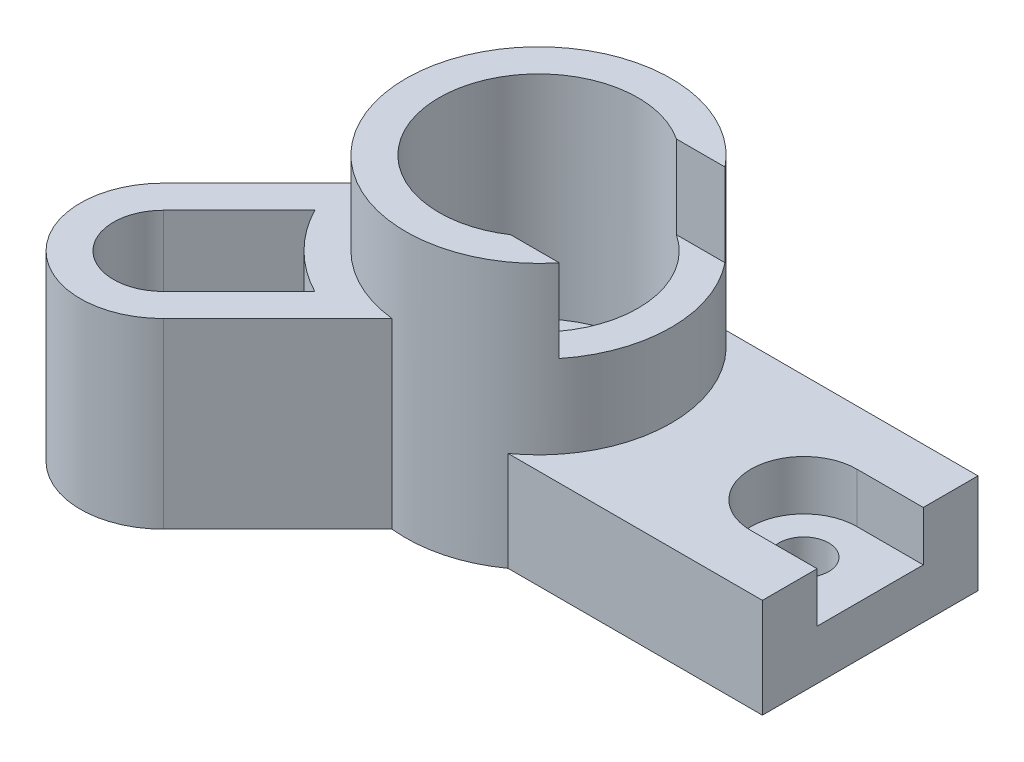
ISO-10303-21;
HEADER;
FILE_DESCRIPTION(('STEP AP214'),'2;1');
FILE_NAME('part.step','',(''),(''),'','','');
FILE_SCHEMA(('AUTOMOTIVE_DESIGN { 1 0 10303 214 1 1 1 1 }'));
ENDSEC;
DATA;
#1=APPLICATION_CONTEXT('core data for automotive mechanical design processes');
#2=APPLICATION_PROTOCOL_DEFINITION('international standard','automotive_design',2000,#1);
#3=PRODUCT_CONTEXT('',#1,'mechanical');
#4=PRODUCT('Part','Part','',(#3));
#5=PRODUCT_RELATED_PRODUCT_CATEGORY('part','',(#4));
#6=PRODUCT_DEFINITION_FORMATION('','',#4);
#7=PRODUCT_DEFINITION_CONTEXT('part definition',#1,'design');
#8=PRODUCT_DEFINITION('design','',#6,#7);
#9=PRODUCT_DEFINITION_SHAPE('','',#8);
#10=(LENGTH_UNIT() NAMED_UNIT(*) SI_UNIT(.MILLI.,.METRE.));
#11=(NAMED_UNIT(*) PLANE_ANGLE_UNIT() SI_UNIT($,.RADIAN.));
#12=(NAMED_UNIT(*) SI_UNIT($,.STERADIAN.) SOLID_ANGLE_UNIT());
#13=UNCERTAINTY_MEASURE_WITH_UNIT(LENGTH_MEASURE(1.E-05),#10,'distance_accuracy_value','');
#14=(GEOMETRIC_REPRESENTATION_CONTEXT(3) GLOBAL_UNCERTAINTY_ASSIGNED_CONTEXT((#13)) GLOBAL_UNIT_ASSIGNED_CONTEXT((#10,
#11,#12)) REPRESENTATION_CONTEXT('',''));
#15=CARTESIAN_POINT('',(0.,0.,0.));
#16=DIRECTION('',(0.,0.,1.));
#17=DIRECTION('',(1.,0.,0.));
#18=AXIS2_PLACEMENT_3D('',#15,#16,#17);
#19=CARTESIAN_POINT('',(0.,80.,0.));
#20=DIRECTION('',(0.,-1.,0.));
#21=DIRECTION('',(0.,0.,-1.));
#22=AXIS2_PLACEMENT_3D('',#19,#20,#21);
#23=CYLINDRICAL_SURFACE('',#22,40.);
#24=DIRECTION('',(0.,-1.,0.));
#25=VECTOR('',#24,1.);
#26=CARTESIAN_POINT('',(23.318447632722,30.,32.5));
#27=LINE('',#26,#25);
#28=CARTESIAN_POINT('',(23.318447632722,30.,32.5));
#29=VERTEX_POINT('',#28);
#30=CARTESIAN_POINT('',(23.318447632722,0.,32.5));
#31=VERTEX_POINT('',#30);
#32=EDGE_CURVE('E302',#29,#31,#27,.T.);
#33=ORIENTED_EDGE('',*,*,#32,.F.);
#34=CARTESIAN_POINT('',(0.,30.,0.));
#35=DIRECTION('',(0.,1.,0.));
#36=DIRECTION('',(0.,0.,1.));
#37=AXIS2_PLACEMENT_3D('',#34,#35,#36);
#38=CIRCLE('',#37,40.);
#39=CARTESIAN_POINT('',(23.318447632722,30.,-32.5));
#40=VERTEX_POINT('',#39);
#41=EDGE_CURVE('E279',#29,#40,#38,.T.);
#42=ORIENTED_EDGE('',*,*,#41,.T.);
#43=DIRECTION('',(0.,-1.,0.));
#44=VECTOR('',#43,1.);
#45=CARTESIAN_POINT('',(23.318447632722,30.,-32.5));
#46=LINE('',#45,#44);
#47=CARTESIAN_POINT('',(23.318447632722,0.,-32.5));
#48=VERTEX_POINT('',#47);
#49=EDGE_CURVE('E289',#40,#48,#46,.T.);
#50=ORIENTED_EDGE('',*,*,#49,.T.);
#51=CARTESIAN_POINT('',(0.,0.,0.));
#52=DIRECTION('',(0.,1.,0.));
#53=DIRECTION('',(0.,0.,1.));
#54=AXIS2_PLACEMENT_3D('',#51,#52,#53);
#55=CIRCLE('',#54,40.);
#56=CARTESIAN_POINT('',(-39.7570716954833,0.,4.40173263615613));
#57=VERTEX_POINT('',#56);
#58=EDGE_CURVE('E332',#48,#57,#55,.T.);
#59=ORIENTED_EDGE('',*,*,#58,.T.);
#60=DIRECTION('',(0.,-1.,0.));
#61=VECTOR('',#60,1.);
#62=CARTESIAN_POINT('',(-39.7570716954833,55.,4.40173263615613));
#63=LINE('',#62,#61);
#64=CARTESIAN_POINT('',(-39.7570716954833,55.,4.40173263615613));
#65=VERTEX_POINT('',#64);
#66=EDGE_CURVE('E335',#65,#57,#63,.T.);
#67=ORIENTED_EDGE('',*,*,#66,.F.);
#68=CARTESIAN_POINT('',(0.,55.,0.));
#69=DIRECTION('',(0.,1.,0.));
#70=DIRECTION('',(0.,0.,1.));
#71=AXIS2_PLACEMENT_3D('',#68,#69,#70);
#72=CIRCLE('',#71,40.);
#73=CARTESIAN_POINT('',(-4.40173263615573,55.,39.7570716954833));
#74=VERTEX_POINT('',#73);
#75=EDGE_CURVE('E310',#65,#74,#72,.T.);
#76=ORIENTED_EDGE('',*,*,#75,.T.);
#77=DIRECTION('',(0.,-1.,0.));
#78=VECTOR('',#77,1.);
#79=CARTESIAN_POINT('',(-4.40173263615573,55.,39.7570716954833));
#80=LINE('',#79,#78);
#81=CARTESIAN_POINT('',(-4.40173263615573,0.,39.7570716954833));
#82=VERTEX_POINT('',#81);
#83=EDGE_CURVE('E316',#74,#82,#80,.T.);
#84=ORIENTED_EDGE('',*,*,#83,.T.);
#85=EDGE_CURVE('E42',#82,#31,#55,.T.);
#86=ORIENTED_EDGE('',*,*,#85,.T.);
#87=EDGE_LOOP('',(#33,#42,#50,#59,#67,#76,#84,#86));
#88=FACE_BOUND('',#87,.T.);
#89=DIRECTION('',(0.,-1.,0.));
#90=VECTOR('',#89,1.);
#91=CARTESIAN_POINT('',(31.224989991992,80.001,25.));
#92=LINE('',#91,#90);
#93=CARTESIAN_POINT('',(31.224989991992,80.,25.));
#94=VERTEX_POINT('',#93);
#95=CARTESIAN_POINT('',(31.224989991992,55.,25.));
#96=VERTEX_POINT('',#95);
#97=EDGE_CURVE('E220',#94,#96,#92,.T.);
#98=ORIENTED_EDGE('',*,*,#97,.F.);
#99=CARTESIAN_POINT('',(0.,80.,0.));
#100=DIRECTION('',(0.,1.,0.));
#101=DIRECTION('',(0.,0.,1.));
#102=AXIS2_PLACEMENT_3D('',#99,#100,#101);
#103=CIRCLE('',#102,40.);
#104=CARTESIAN_POINT('',(31.224989991992,80.,-25.));
#105=VERTEX_POINT('',#104);
#106=EDGE_CURVE('E11',#105,#94,#103,.T.);
#107=ORIENTED_EDGE('',*,*,#106,.F.);
#108=DIRECTION('',(0.,-1.,0.));
#109=VECTOR('',#108,1.);
#110=CARTESIAN_POINT('',(31.224989991992,80.001,-25.));
#111=LINE('',#110,#109);
#112=CARTESIAN_POINT('',(31.224989991992,55.,-25.));
#113=VERTEX_POINT('',#112);
#114=EDGE_CURVE('E213',#105,#113,#111,.T.);
#115=ORIENTED_EDGE('',*,*,#114,.T.);
#116=CARTESIAN_POINT('',(0.,55.,0.));
#117=DIRECTION('',(0.,1.,0.));
#118=DIRECTION('',(0.,0.,1.));
#119=AXIS2_PLACEMENT_3D('',#116,#117,#118);
#120=CIRCLE('',#119,40.);
#121=EDGE_CURVE('E202',#96,#113,#120,.T.);
#122=ORIENTED_EDGE('',*,*,#121,.F.);
#123=EDGE_LOOP('',(#98,#107,#115,#122));
#124=FACE_BOUND('',#123,.T.);
#125=ADVANCED_FACE('F41',(#88,#124),#23,.T.);
#126=CARTESIAN_POINT('',(0.,80.,0.));
#127=DIRECTION('',(0.,1.,0.));
#128=DIRECTION('',(0.,0.,1.));
#129=AXIS2_PLACEMENT_3D('',#126,#127,#128);
#130=PLANE('',#129);
#131=CARTESIAN_POINT('',(0.,80.,0.));
#132=DIRECTION('',(0.,1.,0.));
#133=DIRECTION('',(0.,0.,1.));
#134=AXIS2_PLACEMENT_3D('',#131,#132,#133);
#135=CIRCLE('',#134,30.);
#136=CARTESIAN_POINT('',(16.583123951777,80.,-25.));
#137=VERTEX_POINT('',#136);
#138=CARTESIAN_POINT('',(16.583123951777,80.,25.));
#139=VERTEX_POINT('',#138);
#140=EDGE_CURVE('E176',#137,#139,#135,.T.);
#141=ORIENTED_EDGE('',*,*,#140,.F.);
#142=DIRECTION('',(1.,0.,0.));
#143=VECTOR('',#142,1.);
#144=CARTESIAN_POINT('',(16.583123951777,80.,-25.));
#145=LINE('',#144,#143);
#146=EDGE_CURVE('E205',#137,#105,#145,.T.);
#147=ORIENTED_EDGE('',*,*,#146,.T.);
#148=ORIENTED_EDGE('',*,*,#106,.T.);
#149=DIRECTION('',(1.,0.,0.));
#150=VECTOR('',#149,1.);
#151=CARTESIAN_POINT('',(16.583123951777,80.,25.));
#152=LINE('',#151,#150);
#153=EDGE_CURVE('E195',#139,#94,#152,.T.);
#154=ORIENTED_EDGE('',*,*,#153,.F.);
#155=EDGE_LOOP('',(#141,#147,#148,#154));
#156=FACE_BOUND('',#155,.T.);
#157=ADVANCED_FACE('F199',(#156),#130,.T.);
#158=CARTESIAN_POINT('',(100.,30.,0.));
#159=DIRECTION('',(1.,0.,0.));
#160=DIRECTION('',(0.,0.,-1.));
#161=AXIS2_PLACEMENT_3D('',#158,#159,#160);
#162=PLANE('',#161);
#163=DIRECTION('',(0.,0.,1.));
#164=VECTOR('',#163,1.);
#165=CARTESIAN_POINT('',(100.,15.,0.));
#166=LINE('',#165,#164);
#167=CARTESIAN_POINT('',(100.,15.,-16.));
#168=VERTEX_POINT('',#167);
#169=CARTESIAN_POINT('',(100.,15.,16.));
#170=VERTEX_POINT('',#169);
#171=EDGE_CURVE('E225',#168,#170,#166,.T.);
#172=ORIENTED_EDGE('',*,*,#171,.T.);
#173=DIRECTION('',(0.,1.,0.));
#174=VECTOR('',#173,1.);
#175=CARTESIAN_POINT('',(100.,15.,16.));
#176=LINE('',#175,#174);
#177=CARTESIAN_POINT('',(100.,30.,16.));
#178=VERTEX_POINT('',#177);
#179=EDGE_CURVE('E241',#170,#178,#176,.T.);
#180=ORIENTED_EDGE('',*,*,#179,.T.);
#181=DIRECTION('',(0.,0.,1.));
#182=VECTOR('',#181,1.);
#183=CARTESIAN_POINT('',(100.,30.,0.));
#184=LINE('',#183,#182);
#185=CARTESIAN_POINT('',(100.,30.,32.5));
#186=VERTEX_POINT('',#185);
#187=EDGE_CURVE('E283',#178,#186,#184,.T.);
#188=ORIENTED_EDGE('',*,*,#187,.T.);
#189=DIRECTION('',(0.,-1.,0.));
#190=VECTOR('',#189,1.);
#191=CARTESIAN_POINT('',(100.,30.,32.5));
#192=LINE('',#191,#190);
#193=CARTESIAN_POINT('',(100.,0.,32.5));
#194=VERTEX_POINT('',#193);
#195=EDGE_CURVE('E305',#186,#194,#192,.T.);
#196=ORIENTED_EDGE('',*,*,#195,.T.);
#197=DIRECTION('',(0.,0.,1.));
#198=VECTOR('',#197,1.);
#199=CARTESIAN_POINT('',(100.,0.,0.));
#200=LINE('',#199,#198);
#201=CARTESIAN_POINT('',(100.,0.,-32.5));
#202=VERTEX_POINT('',#201);
#203=EDGE_CURVE('E291',#202,#194,#200,.T.);
#204=ORIENTED_EDGE('',*,*,#203,.F.);
#205=DIRECTION('',(0.,-1.,0.));
#206=VECTOR('',#205,1.);
#207=CARTESIAN_POINT('',(100.,30.,-32.5));
#208=LINE('',#207,#206);
#209=CARTESIAN_POINT('',(100.,30.,-32.5));
#210=VERTEX_POINT('',#209);
#211=EDGE_CURVE('E297',#210,#202,#208,.T.);
#212=ORIENTED_EDGE('',*,*,#211,.F.);
#213=CARTESIAN_POINT('',(100.,30.,-16.));
#214=VERTEX_POINT('',#213);
#215=EDGE_CURVE('E282',#210,#214,#184,.T.);
#216=ORIENTED_EDGE('',*,*,#215,.T.);
#217=DIRECTION('',(0.,1.,0.));
#218=VECTOR('',#217,1.);
#219=CARTESIAN_POINT('',(100.,15.,-16.));
#220=LINE('',#219,#218);
#221=EDGE_CURVE('E242',#168,#214,#220,.T.);
#222=ORIENTED_EDGE('',*,*,#221,.F.);
#223=EDGE_LOOP('',(#172,#180,#188,#196,#204,#212,#216,#222));
#224=FACE_BOUND('',#223,.T.);
#225=ADVANCED_FACE('F386',(#224),#162,.T.);
#226=CARTESIAN_POINT('',(0.,30.,0.));
#227=DIRECTION('',(0.,1.,0.));
#228=DIRECTION('',(0.,0.,1.));
#229=AXIS2_PLACEMENT_3D('',#226,#227,#228);
#230=PLANE('',#229);
#231=CARTESIAN_POINT('',(80.,30.,0.));
#232=DIRECTION('',(0.,1.,0.));
#233=DIRECTION('',(0.,0.,1.));
#234=AXIS2_PLACEMENT_3D('',#231,#232,#233);
#235=CIRCLE('',#234,16.);
#236=CARTESIAN_POINT('',(80.,30.,-16.));
#237=VERTEX_POINT('',#236);
#238=CARTESIAN_POINT('',(80.,30.,16.));
#239=VERTEX_POINT('',#238);
#240=EDGE_CURVE('E223',#237,#239,#235,.T.);
#241=ORIENTED_EDGE('',*,*,#240,.F.);
#242=DIRECTION('',(1.,0.,0.));
#243=VECTOR('',#242,1.);
#244=CARTESIAN_POINT('',(0.,30.,-16.));
#245=LINE('',#244,#243);
#246=EDGE_CURVE('E54',#237,#214,#245,.T.);
#247=ORIENTED_EDGE('',*,*,#246,.T.);
#248=ORIENTED_EDGE('',*,*,#215,.F.);
#249=DIRECTION('',(1.,0.,0.));
#250=VECTOR('',#249,1.);
#251=CARTESIAN_POINT('',(0.,30.,-32.4999999999999));
#252=LINE('',#251,#250);
#253=EDGE_CURVE('E290',#40,#210,#252,.T.);
#254=ORIENTED_EDGE('',*,*,#253,.F.);
#255=ORIENTED_EDGE('',*,*,#41,.F.);
#256=DIRECTION('',(1.,0.,0.));
#257=VECTOR('',#256,1.);
#258=CARTESIAN_POINT('',(0.,30.,32.5));
#259=LINE('',#258,#257);
#260=EDGE_CURVE('E278',#29,#186,#259,.T.);
#261=ORIENTED_EDGE('',*,*,#260,.T.);
#262=ORIENTED_EDGE('',*,*,#187,.F.);
#263=DIRECTION('',(1.,0.,0.));
#264=VECTOR('',#263,1.);
#265=CARTESIAN_POINT('',(0.,30.,16.));
#266=LINE('',#265,#264);
#267=EDGE_CURVE('E234',#239,#178,#266,.T.);
#268=ORIENTED_EDGE('',*,*,#267,.F.);
#269=EDGE_LOOP('',(#241,#247,#248,#254,#255,#261,#262,#268));
#270=FACE_BOUND('',#269,.T.);
#271=ADVANCED_FACE('F357',(#270),#230,.T.);
#272=CARTESIAN_POINT('',(0.,0.,0.));
#273=DIRECTION('',(0.,1.,0.));
#274=DIRECTION('',(0.,0.,1.));
#275=AXIS2_PLACEMENT_3D('',#272,#273,#274);
#276=PLANE('',#275);
#277=CARTESIAN_POINT('',(-56.5685424949235,0.,56.5685424949241));
#278=DIRECTION('',(0.,-1.,0.));
#279=DIRECTION('',(0.,0.,-1.));
#280=AXIS2_PLACEMENT_3D('',#277,#278,#279);
#281=CIRCLE('',#280,10.);
#282=CARTESIAN_POINT('',(-56.5685424949235,0.,46.5685424949241));
#283=VERTEX_POINT('',#282);
#284=EDGE_CURVE('E186',#283,#283,#281,.T.);
#285=ORIENTED_EDGE('',*,*,#284,.F.);
#286=EDGE_LOOP('',(#285));
#287=FACE_BOUND('',#286,.T.);
#288=CARTESIAN_POINT('',(80.,0.,0.));
#289=DIRECTION('',(0.,-1.,0.));
#290=DIRECTION('',(0.,0.,-1.));
#291=AXIS2_PLACEMENT_3D('',#288,#289,#290);
#292=CIRCLE('',#291,7.5);
#293=CARTESIAN_POINT('',(80.,0.,-7.5));
#294=VERTEX_POINT('',#293);
#295=EDGE_CURVE('E411',#294,#294,#292,.T.);
#296=ORIENTED_EDGE('',*,*,#295,.F.);
#297=EDGE_LOOP('',(#296));
#298=FACE_BOUND('',#297,.T.);
#299=CARTESIAN_POINT('',(0.,0.,0.));
#300=DIRECTION('',(0.,-1.,0.));
#301=DIRECTION('',(0.,0.,-1.));
#302=AXIS2_PLACEMENT_3D('',#299,#300,#301);
#303=CIRCLE('',#302,20.);
#304=CARTESIAN_POINT('',(0.,0.,-20.));
#305=VERTEX_POINT('',#304);
#306=EDGE_CURVE('E412',#305,#305,#303,.T.);
#307=ORIENTED_EDGE('',*,*,#306,.F.);
#308=EDGE_LOOP('',(#307));
#309=FACE_BOUND('',#308,.T.);
#310=ORIENTED_EDGE('',*,*,#85,.F.);
#311=DIRECTION('',(0.707106781186544,0.,-0.707106781186551));
#312=VECTOR('',#311,1.);
#313=CARTESIAN_POINT('',(17.6776695296638,0.,17.6776695296636));
#314=LINE('',#313,#312);
#315=CARTESIAN_POINT('',(-38.8908729652597,0.,74.2462120245877));
#316=VERTEX_POINT('',#315);
#317=EDGE_CURVE('E311',#316,#82,#314,.T.);
#318=ORIENTED_EDGE('',*,*,#317,.F.);
#319=CARTESIAN_POINT('',(-56.5685424949235,0.,56.5685424949241));
#320=DIRECTION('',(0.,1.,0.));
#321=DIRECTION('',(0.,0.,1.));
#322=AXIS2_PLACEMENT_3D('',#319,#320,#321);
#323=CIRCLE('',#322,25.);
#324=CARTESIAN_POINT('',(-74.2462120245873,0.,38.8908729652605));
#325=VERTEX_POINT('',#324);
#326=EDGE_CURVE('E321',#325,#316,#323,.T.);
#327=ORIENTED_EDGE('',*,*,#326,.F.);
#328=DIRECTION('',(0.707106781186544,0.,-0.707106781186551));
#329=VECTOR('',#328,1.);
#330=CARTESIAN_POINT('',(-17.6776695296638,0.,-17.6776695296636));
#331=LINE('',#330,#329);
#332=EDGE_CURVE('E306',#325,#57,#331,.T.);
#333=ORIENTED_EDGE('',*,*,#332,.T.);
#334=ORIENTED_EDGE('',*,*,#58,.F.);
#335=DIRECTION('',(1.,0.,0.));
#336=VECTOR('',#335,1.);
#337=CARTESIAN_POINT('',(0.,0.,-32.4999999999999));
#338=LINE('',#337,#336);
#339=EDGE_CURVE('E277',#48,#202,#338,.T.);
#340=ORIENTED_EDGE('',*,*,#339,.T.);
#341=ORIENTED_EDGE('',*,*,#203,.T.);
#342=DIRECTION('',(1.,0.,0.));
#343=VECTOR('',#342,1.);
#344=CARTESIAN_POINT('',(0.,0.,32.5));
#345=LINE('',#344,#343);
#346=EDGE_CURVE('E269',#31,#194,#345,.T.);
#347=ORIENTED_EDGE('',*,*,#346,.F.);
#348=EDGE_LOOP('',(#310,#318,#327,#333,#334,#340,#341,#347));
#349=FACE_BOUND('',#348,.T.);
#350=ADVANCED_FACE('F350',(#287,#298,#309,#349),#276,.F.);
#351=CARTESIAN_POINT('',(-17.6776695296638,55.,-17.6776695296636));
#352=DIRECTION('',(-0.707106781186551,0.,-0.707106781186544));
#353=DIRECTION('',(-0.707106781186544,0.,0.707106781186551));
#354=AXIS2_PLACEMENT_3D('',#351,#352,#353);
#355=PLANE('',#354);
#356=ORIENTED_EDGE('',*,*,#332,.F.);
#357=DIRECTION('',(0.,-1.,0.));
#358=VECTOR('',#357,1.);
#359=CARTESIAN_POINT('',(-74.2462120245873,55.,38.8908729652605));
#360=LINE('',#359,#358);
#361=CARTESIAN_POINT('',(-74.2462120245873,55.,38.8908729652605));
#362=VERTEX_POINT('',#361);
#363=EDGE_CURVE('E329',#362,#325,#360,.T.);
#364=ORIENTED_EDGE('',*,*,#363,.F.);
#365=DIRECTION('',(0.707106781186544,0.,-0.707106781186551));
#366=VECTOR('',#365,1.);
#367=CARTESIAN_POINT('',(-17.6776695296638,55.,-17.6776695296636));
#368=LINE('',#367,#366);
#369=EDGE_CURVE('E309',#362,#65,#368,.T.);
#370=ORIENTED_EDGE('',*,*,#369,.T.);
#371=ORIENTED_EDGE('',*,*,#66,.T.);
#372=EDGE_LOOP('',(#356,#364,#370,#371));
#373=FACE_BOUND('',#372,.T.);
#374=ADVANCED_FACE('F363',(#373),#355,.T.);
#375=CARTESIAN_POINT('',(-56.5685424949235,55.,56.5685424949241));
#376=DIRECTION('',(0.,-1.,0.));
#377=DIRECTION('',(0.,0.,-1.));
#378=AXIS2_PLACEMENT_3D('',#375,#376,#377);
#379=CYLINDRICAL_SURFACE('',#378,25.);
#380=ORIENTED_EDGE('',*,*,#326,.T.);
#381=DIRECTION('',(0.,-1.,0.));
#382=VECTOR('',#381,1.);
#383=CARTESIAN_POINT('',(-38.8908729652597,55.,74.2462120245877));
#384=LINE('',#383,#382);
#385=CARTESIAN_POINT('',(-38.8908729652597,55.,74.2462120245877));
#386=VERTEX_POINT('',#385);
#387=EDGE_CURVE('E330',#386,#316,#384,.T.);
#388=ORIENTED_EDGE('',*,*,#387,.F.);
#389=CARTESIAN_POINT('',(-56.5685424949235,55.,56.5685424949241));
#390=DIRECTION('',(0.,1.,0.));
#391=DIRECTION('',(0.,0.,1.));
#392=AXIS2_PLACEMENT_3D('',#389,#390,#391);
#393=CIRCLE('',#392,25.);
#394=EDGE_CURVE('E313',#362,#386,#393,.T.);
#395=ORIENTED_EDGE('',*,*,#394,.F.);
#396=ORIENTED_EDGE('',*,*,#363,.T.);
#397=EDGE_LOOP('',(#380,#388,#395,#396));
#398=FACE_BOUND('',#397,.T.);
#399=ADVANCED_FACE('F366',(#398),#379,.T.);
#400=CARTESIAN_POINT('',(17.6776695296638,55.,17.6776695296636));
#401=DIRECTION('',(-0.707106781186552,0.,-0.707106781186544));
#402=DIRECTION('',(-0.707106781186544,0.,0.707106781186551));
#403=AXIS2_PLACEMENT_3D('',#400,#401,#402);
#404=PLANE('',#403);
#405=ORIENTED_EDGE('',*,*,#317,.T.);
#406=ORIENTED_EDGE('',*,*,#83,.F.);
#407=DIRECTION('',(0.707106781186544,0.,-0.707106781186551));
#408=VECTOR('',#407,1.);
#409=CARTESIAN_POINT('',(17.6776695296638,55.,17.6776695296636));
#410=LINE('',#409,#408);
#411=EDGE_CURVE('E317',#386,#74,#410,.T.);
#412=ORIENTED_EDGE('',*,*,#411,.F.);
#413=ORIENTED_EDGE('',*,*,#387,.T.);
#414=EDGE_LOOP('',(#405,#406,#412,#413));
#415=FACE_BOUND('',#414,.T.);
#416=ADVANCED_FACE('F371',(#415),#404,.F.);
#417=CARTESIAN_POINT('',(0.,55.,0.));
#418=DIRECTION('',(0.,1.,0.));
#419=DIRECTION('',(0.,0.,1.));
#420=AXIS2_PLACEMENT_3D('',#417,#418,#419);
#421=PLANE('',#420);
#422=DIRECTION('',(-0.707106781186544,0.,0.707106781186551));
#423=VECTOR('',#422,1.);
#424=CARTESIAN_POINT('',(-10.6066017177983,55.,-10.6066017177982));
#425=LINE('',#424,#423);
#426=CARTESIAN_POINT('',(-44.3334456258782,55.,23.1202421902821));
#427=VERTEX_POINT('',#426);
#428=CARTESIAN_POINT('',(-67.1751442127218,55.,45.9619407771259));
#429=VERTEX_POINT('',#428);
#430=EDGE_CURVE('E65',#427,#429,#425,.T.);
#431=ORIENTED_EDGE('',*,*,#430,.F.);
#432=CARTESIAN_POINT('',(0.,55.,0.));
#433=DIRECTION('',(0.,1.,0.));
#434=DIRECTION('',(0.,0.,1.));
#435=AXIS2_PLACEMENT_3D('',#432,#433,#434);
#436=CIRCLE('',#435,50.);
#437=CARTESIAN_POINT('',(-23.1202421902817,55.,44.3334456258784));
#438=VERTEX_POINT('',#437);
#439=EDGE_CURVE('E249',#427,#438,#436,.T.);
#440=ORIENTED_EDGE('',*,*,#439,.T.);
#441=DIRECTION('',(0.707106781186544,0.,-0.707106781186551));
#442=VECTOR('',#441,1.);
#443=CARTESIAN_POINT('',(10.6066017177983,55.,10.6066017177981));
#444=LINE('',#443,#442);
#445=CARTESIAN_POINT('',(-45.9619407771252,55.,67.1751442127222));
#446=VERTEX_POINT('',#445);
#447=EDGE_CURVE('E263',#446,#438,#444,.T.);
#448=ORIENTED_EDGE('',*,*,#447,.F.);
#449=CARTESIAN_POINT('',(-56.5685424949235,55.,56.5685424949241));
#450=DIRECTION('',(0.,1.,0.));
#451=DIRECTION('',(0.,0.,1.));
#452=AXIS2_PLACEMENT_3D('',#449,#450,#451);
#453=CIRCLE('',#452,15.);
#454=EDGE_CURVE('E257',#429,#446,#453,.T.);
#455=ORIENTED_EDGE('',*,*,#454,.F.);
#456=EDGE_LOOP('',(#431,#440,#448,#455));
#457=FACE_BOUND('',#456,.T.);
#458=ORIENTED_EDGE('',*,*,#75,.F.);
#459=ORIENTED_EDGE('',*,*,#369,.F.);
#460=ORIENTED_EDGE('',*,*,#394,.T.);
#461=ORIENTED_EDGE('',*,*,#411,.T.);
#462=EDGE_LOOP('',(#458,#459,#460,#461));
#463=FACE_BOUND('',#462,.T.);
#464=ADVANCED_FACE('F367',(#457,#463),#421,.T.);
#465=CARTESIAN_POINT('',(0.,30.,32.5));
#466=DIRECTION('',(0.,0.,-1.));
#467=DIRECTION('',(-1.,0.,0.));
#468=AXIS2_PLACEMENT_3D('',#465,#466,#467);
#469=PLANE('',#468);
#470=ORIENTED_EDGE('',*,*,#346,.T.);
#471=ORIENTED_EDGE('',*,*,#195,.F.);
#472=ORIENTED_EDGE('',*,*,#260,.F.);
#473=ORIENTED_EDGE('',*,*,#32,.T.);
#474=EDGE_LOOP('',(#470,#471,#472,#473));
#475=FACE_BOUND('',#474,.T.);
#476=ADVANCED_FACE('F355',(#475),#469,.F.);
#477=CARTESIAN_POINT('',(0.,30.,-32.4999999999999));
#478=DIRECTION('',(0.,0.,-1.));
#479=DIRECTION('',(-1.,0.,0.));
#480=AXIS2_PLACEMENT_3D('',#477,#478,#479);
#481=PLANE('',#480);
#482=ORIENTED_EDGE('',*,*,#339,.F.);
#483=ORIENTED_EDGE('',*,*,#49,.F.);
#484=ORIENTED_EDGE('',*,*,#253,.T.);
#485=ORIENTED_EDGE('',*,*,#211,.T.);
#486=EDGE_LOOP('',(#482,#483,#484,#485));
#487=FACE_BOUND('',#486,.T.);
#488=ADVANCED_FACE('F472',(#487),#481,.T.);
#489=CARTESIAN_POINT('',(-10.6066017177983,30.,-10.6066017177982));
#490=DIRECTION('',(-0.707106781186551,0.,-0.707106781186544));
#491=DIRECTION('',(-0.707106781186544,0.,0.707106781186551));
#492=AXIS2_PLACEMENT_3D('',#489,#490,#491);
#493=PLANE('',#492);
#494=ORIENTED_EDGE('',*,*,#430,.T.);
#495=DIRECTION('',(0.,1.,0.));
#496=VECTOR('',#495,1.);
#497=CARTESIAN_POINT('',(-67.1751442127218,30.,45.9619407771259));
#498=LINE('',#497,#496);
#499=CARTESIAN_POINT('',(-67.1751442127218,30.,45.9619407771259));
#500=VERTEX_POINT('',#499);
#501=EDGE_CURVE('E260',#500,#429,#498,.T.);
#502=ORIENTED_EDGE('',*,*,#501,.F.);
#503=DIRECTION('',(-0.707106781186544,0.,0.707106781186551));
#504=VECTOR('',#503,1.);
#505=CARTESIAN_POINT('',(-10.6066017177983,30.,-10.6066017177982));
#506=LINE('',#505,#504);
#507=CARTESIAN_POINT('',(-44.3334456258782,30.,23.1202421902821));
#508=VERTEX_POINT('',#507);
#509=EDGE_CURVE('E246',#508,#500,#506,.T.);
#510=ORIENTED_EDGE('',*,*,#509,.F.);
#511=DIRECTION('',(0.,1.,0.));
#512=VECTOR('',#511,1.);
#513=CARTESIAN_POINT('',(-44.3334456258782,30.,23.1202421902821));
#514=LINE('',#513,#512);
#515=EDGE_CURVE('E268',#508,#427,#514,.T.);
#516=ORIENTED_EDGE('',*,*,#515,.T.);
#517=EDGE_LOOP('',(#494,#502,#510,#516));
#518=FACE_BOUND('',#517,.T.);
#519=ADVANCED_FACE('F467',(#518),#493,.F.);
#520=CARTESIAN_POINT('',(0.,30.,0.));
#521=DIRECTION('',(0.,1.,0.));
#522=DIRECTION('',(0.,0.,1.));
#523=AXIS2_PLACEMENT_3D('',#520,#521,#522);
#524=CYLINDRICAL_SURFACE('',#523,50.);
#525=ORIENTED_EDGE('',*,*,#439,.F.);
#526=ORIENTED_EDGE('',*,*,#515,.F.);
#527=CARTESIAN_POINT('',(0.,30.,0.));
#528=DIRECTION('',(0.,1.,0.));
#529=DIRECTION('',(0.,0.,1.));
#530=AXIS2_PLACEMENT_3D('',#527,#528,#529);
#531=CIRCLE('',#530,50.);
#532=CARTESIAN_POINT('',(-23.1202421902817,30.,44.3334456258784));
#533=VERTEX_POINT('',#532);
#534=EDGE_CURVE('E259',#508,#533,#531,.T.);
#535=ORIENTED_EDGE('',*,*,#534,.T.);
#536=DIRECTION('',(0.,1.,0.));
#537=VECTOR('',#536,1.);
#538=CARTESIAN_POINT('',(-23.1202421902817,30.,44.3334456258784));
#539=LINE('',#538,#537);
#540=EDGE_CURVE('E272',#533,#438,#539,.T.);
#541=ORIENTED_EDGE('',*,*,#540,.T.);
#542=EDGE_LOOP('',(#525,#526,#535,#541));
#543=FACE_BOUND('',#542,.T.);
#544=ADVANCED_FACE('F465',(#543),#524,.T.);
#545=CARTESIAN_POINT('',(10.6066017177983,30.,10.6066017177981));
#546=DIRECTION('',(0.707106781186551,0.,0.707106781186544));
#547=DIRECTION('',(0.707106781186544,0.,-0.707106781186551));
#548=AXIS2_PLACEMENT_3D('',#545,#546,#547);
#549=PLANE('',#548);
#550=ORIENTED_EDGE('',*,*,#447,.T.);
#551=ORIENTED_EDGE('',*,*,#540,.F.);
#552=DIRECTION('',(0.707106781186544,0.,-0.707106781186551));
#553=VECTOR('',#552,1.);
#554=CARTESIAN_POINT('',(10.6066017177983,30.,10.6066017177981));
#555=LINE('',#554,#553);
#556=CARTESIAN_POINT('',(-45.9619407771252,30.,67.1751442127222));
#557=VERTEX_POINT('',#556);
#558=EDGE_CURVE('E254',#557,#533,#555,.T.);
#559=ORIENTED_EDGE('',*,*,#558,.F.);
#560=DIRECTION('',(0.,1.,0.));
#561=VECTOR('',#560,1.);
#562=CARTESIAN_POINT('',(-45.9619407771252,30.,67.1751442127222));
#563=LINE('',#562,#561);
#564=EDGE_CURVE('E271',#557,#446,#563,.T.);
#565=ORIENTED_EDGE('',*,*,#564,.T.);
#566=EDGE_LOOP('',(#550,#551,#559,#565));
#567=FACE_BOUND('',#566,.T.);
#568=ADVANCED_FACE('F464',(#567),#549,.F.);
#569=CARTESIAN_POINT('',(-56.5685424949235,30.,56.5685424949241));
#570=DIRECTION('',(0.,1.,0.));
#571=DIRECTION('',(0.,0.,1.));
#572=AXIS2_PLACEMENT_3D('',#569,#570,#571);
#573=CYLINDRICAL_SURFACE('',#572,15.);
#574=ORIENTED_EDGE('',*,*,#454,.T.);
#575=ORIENTED_EDGE('',*,*,#564,.F.);
#576=CARTESIAN_POINT('',(-56.5685424949235,30.,56.5685424949241));
#577=DIRECTION('',(0.,1.,0.));
#578=DIRECTION('',(0.,0.,1.));
#579=AXIS2_PLACEMENT_3D('',#576,#577,#578);
#580=CIRCLE('',#579,15.);
#581=EDGE_CURVE('E248',#500,#557,#580,.T.);
#582=ORIENTED_EDGE('',*,*,#581,.F.);
#583=ORIENTED_EDGE('',*,*,#501,.T.);
#584=EDGE_LOOP('',(#574,#575,#582,#583));
#585=FACE_BOUND('',#584,.T.);
#586=ADVANCED_FACE('F459',(#585),#573,.F.);
#587=CARTESIAN_POINT('',(0.,30.,0.));
#588=DIRECTION('',(0.,1.,0.));
#589=DIRECTION('',(0.,0.,1.));
#590=AXIS2_PLACEMENT_3D('',#587,#588,#589);
#591=PLANE('',#590);
#592=CARTESIAN_POINT('',(-56.5685424949235,30.,56.5685424949241));
#593=DIRECTION('',(0.,1.,0.));
#594=DIRECTION('',(0.,0.,1.));
#595=AXIS2_PLACEMENT_3D('',#592,#593,#594);
#596=CIRCLE('',#595,10.);
#597=CARTESIAN_POINT('',(-56.5685424949235,30.,66.5685424949241));
#598=VERTEX_POINT('',#597);
#599=EDGE_CURVE('E613',#598,#598,#596,.F.);
#600=ORIENTED_EDGE('',*,*,#599,.T.);
#601=EDGE_LOOP('',(#600));
#602=FACE_BOUND('',#601,.T.);
#603=ORIENTED_EDGE('',*,*,#509,.T.);
#604=ORIENTED_EDGE('',*,*,#581,.T.);
#605=ORIENTED_EDGE('',*,*,#558,.T.);
#606=ORIENTED_EDGE('',*,*,#534,.F.);
#607=EDGE_LOOP('',(#603,#604,#605,#606));
#608=FACE_BOUND('',#607,.T.);
#609=ADVANCED_FACE('F458',(#602,#608),#591,.T.);
#610=CARTESIAN_POINT('',(0.,15.,-16.));
#611=DIRECTION('',(0.,0.,1.));
#612=DIRECTION('',(1.,0.,0.));
#613=AXIS2_PLACEMENT_3D('',#610,#611,#612);
#614=PLANE('',#613);
#615=ORIENTED_EDGE('',*,*,#246,.F.);
#616=DIRECTION('',(0.,1.,0.));
#617=VECTOR('',#616,1.);
#618=CARTESIAN_POINT('',(80.,15.,-16.));
#619=LINE('',#618,#617);
#620=CARTESIAN_POINT('',(80.,15.,-16.));
#621=VERTEX_POINT('',#620);
#622=EDGE_CURVE('E235',#621,#237,#619,.T.);
#623=ORIENTED_EDGE('',*,*,#622,.F.);
#624=DIRECTION('',(1.,0.,0.));
#625=VECTOR('',#624,1.);
#626=CARTESIAN_POINT('',(0.,15.,-16.));
#627=LINE('',#626,#625);
#628=EDGE_CURVE('E217',#621,#168,#627,.T.);
#629=ORIENTED_EDGE('',*,*,#628,.T.);
#630=ORIENTED_EDGE('',*,*,#221,.T.);
#631=EDGE_LOOP('',(#615,#623,#629,#630));
#632=FACE_BOUND('',#631,.T.);
#633=ADVANCED_FACE('F453',(#632),#614,.T.);
#634=CARTESIAN_POINT('',(0.,15.,16.));
#635=DIRECTION('',(0.,0.,1.));
#636=DIRECTION('',(1.,0.,0.));
#637=AXIS2_PLACEMENT_3D('',#634,#635,#636);
#638=PLANE('',#637);
#639=ORIENTED_EDGE('',*,*,#267,.T.);
#640=ORIENTED_EDGE('',*,*,#179,.F.);
#641=DIRECTION('',(1.,0.,0.));
#642=VECTOR('',#641,1.);
#643=CARTESIAN_POINT('',(0.,15.,16.));
#644=LINE('',#643,#642);
#645=CARTESIAN_POINT('',(80.,15.,16.));
#646=VERTEX_POINT('',#645);
#647=EDGE_CURVE('E228',#646,#170,#644,.T.);
#648=ORIENTED_EDGE('',*,*,#647,.F.);
#649=DIRECTION('',(0.,1.,0.));
#650=VECTOR('',#649,1.);
#651=CARTESIAN_POINT('',(80.,15.,16.));
#652=LINE('',#651,#650);
#653=EDGE_CURVE('E237',#646,#239,#652,.T.);
#654=ORIENTED_EDGE('',*,*,#653,.T.);
#655=EDGE_LOOP('',(#639,#640,#648,#654));
#656=FACE_BOUND('',#655,.T.);
#657=ADVANCED_FACE('F448',(#656),#638,.F.);
#658=CARTESIAN_POINT('',(80.,15.,0.));
#659=DIRECTION('',(0.,1.,0.));
#660=DIRECTION('',(0.,0.,1.));
#661=AXIS2_PLACEMENT_3D('',#658,#659,#660);
#662=CYLINDRICAL_SURFACE('',#661,16.);
#663=ORIENTED_EDGE('',*,*,#240,.T.);
#664=ORIENTED_EDGE('',*,*,#653,.F.);
#665=CARTESIAN_POINT('',(80.,15.,0.));
#666=DIRECTION('',(0.,1.,0.));
#667=DIRECTION('',(0.,0.,1.));
#668=AXIS2_PLACEMENT_3D('',#665,#666,#667);
#669=CIRCLE('',#668,16.);
#670=EDGE_CURVE('E230',#621,#646,#669,.T.);
#671=ORIENTED_EDGE('',*,*,#670,.F.);
#672=ORIENTED_EDGE('',*,*,#622,.T.);
#673=EDGE_LOOP('',(#663,#664,#671,#672));
#674=FACE_BOUND('',#673,.T.);
#675=ADVANCED_FACE('F450',(#674),#662,.F.);
#676=CARTESIAN_POINT('',(80.,15.,0.));
#677=DIRECTION('',(0.,1.,0.));
#678=DIRECTION('',(0.,0.,1.));
#679=AXIS2_PLACEMENT_3D('',#676,#677,#678);
#680=PLANE('',#679);
#681=CARTESIAN_POINT('',(80.,15.,0.));
#682=DIRECTION('',(0.,1.,0.));
#683=DIRECTION('',(0.,0.,1.));
#684=AXIS2_PLACEMENT_3D('',#681,#682,#683);
#685=CIRCLE('',#684,7.5);
#686=CARTESIAN_POINT('',(80.,15.,7.5));
#687=VERTEX_POINT('',#686);
#688=EDGE_CURVE('E614',#687,#687,#685,.F.);
#689=ORIENTED_EDGE('',*,*,#688,.T.);
#690=EDGE_LOOP('',(#689));
#691=FACE_BOUND('',#690,.T.);
#692=ORIENTED_EDGE('',*,*,#628,.F.);
#693=ORIENTED_EDGE('',*,*,#670,.T.);
#694=ORIENTED_EDGE('',*,*,#647,.T.);
#695=ORIENTED_EDGE('',*,*,#171,.F.);
#696=EDGE_LOOP('',(#692,#693,#694,#695));
#697=FACE_BOUND('',#696,.T.);
#698=ADVANCED_FACE('F443',(#691,#697),#680,.T.);
#699=CARTESIAN_POINT('',(16.583123951777,80.001,25.));
#700=DIRECTION('',(0.,0.,-1.));
#701=DIRECTION('',(-1.,0.,0.));
#702=AXIS2_PLACEMENT_3D('',#699,#700,#701);
#703=PLANE('',#702);
#704=ORIENTED_EDGE('',*,*,#153,.T.);
#705=ORIENTED_EDGE('',*,*,#97,.T.);
#706=DIRECTION('',(1.,0.,0.));
#707=VECTOR('',#706,1.);
#708=CARTESIAN_POINT('',(16.583123951777,55.,25.));
#709=LINE('',#708,#707);
#710=CARTESIAN_POINT('',(16.583123951777,55.,25.));
#711=VERTEX_POINT('',#710);
#712=EDGE_CURVE('E196',#711,#96,#709,.T.);
#713=ORIENTED_EDGE('',*,*,#712,.F.);
#714=DIRECTION('',(0.,-1.,0.));
#715=VECTOR('',#714,1.);
#716=CARTESIAN_POINT('',(16.583123951777,80.001,25.));
#717=LINE('',#716,#715);
#718=EDGE_CURVE('E179',#139,#711,#717,.T.);
#719=ORIENTED_EDGE('',*,*,#718,.F.);
#720=EDGE_LOOP('',(#704,#705,#713,#719));
#721=FACE_BOUND('',#720,.T.);
#722=ADVANCED_FACE('F191',(#721),#703,.T.);
#723=CARTESIAN_POINT('',(16.583123951777,80.001,-25.));
#724=DIRECTION('',(0.,0.,-1.));
#725=DIRECTION('',(-1.,0.,0.));
#726=AXIS2_PLACEMENT_3D('',#723,#724,#725);
#727=PLANE('',#726);
#728=DIRECTION('',(0.,-1.,0.));
#729=VECTOR('',#728,1.);
#730=CARTESIAN_POINT('',(16.583123951777,80.001,-25.));
#731=LINE('',#730,#729);
#732=CARTESIAN_POINT('',(16.583123951777,55.,-25.));
#733=VERTEX_POINT('',#732);
#734=EDGE_CURVE('E182',#137,#733,#731,.T.);
#735=ORIENTED_EDGE('',*,*,#734,.T.);
#736=DIRECTION('',(1.,0.,0.));
#737=VECTOR('',#736,1.);
#738=CARTESIAN_POINT('',(16.583123951777,55.,-25.));
#739=LINE('',#738,#737);
#740=EDGE_CURVE('E209',#733,#113,#739,.T.);
#741=ORIENTED_EDGE('',*,*,#740,.T.);
#742=ORIENTED_EDGE('',*,*,#114,.F.);
#743=ORIENTED_EDGE('',*,*,#146,.F.);
#744=EDGE_LOOP('',(#735,#741,#742,#743));
#745=FACE_BOUND('',#744,.T.);
#746=ADVANCED_FACE('F434',(#745),#727,.F.);
#747=CARTESIAN_POINT('',(0.,55.,0.));
#748=DIRECTION('',(0.,1.,0.));
#749=DIRECTION('',(0.,0.,1.));
#750=AXIS2_PLACEMENT_3D('',#747,#748,#749);
#751=PLANE('',#750);
#752=ORIENTED_EDGE('',*,*,#712,.T.);
#753=ORIENTED_EDGE('',*,*,#121,.T.);
#754=ORIENTED_EDGE('',*,*,#740,.F.);
#755=CARTESIAN_POINT('',(0.,55.,0.));
#756=DIRECTION('',(0.,1.,0.));
#757=DIRECTION('',(0.,0.,1.));
#758=AXIS2_PLACEMENT_3D('',#755,#756,#757);
#759=CIRCLE('',#758,30.);
#760=EDGE_CURVE('E198',#711,#733,#759,.T.);
#761=ORIENTED_EDGE('',*,*,#760,.F.);
#762=EDGE_LOOP('',(#752,#753,#754,#761));
#763=FACE_BOUND('',#762,.T.);
#764=ADVANCED_FACE('F428',(#763),#751,.T.);
#765=CARTESIAN_POINT('',(0.,16.,0.));
#766=DIRECTION('',(0.,1.,0.));
#767=DIRECTION('',(0.,0.,1.));
#768=AXIS2_PLACEMENT_3D('',#765,#766,#767);
#769=CYLINDRICAL_SURFACE('',#768,30.);
#770=ORIENTED_EDGE('',*,*,#718,.T.);
#771=ORIENTED_EDGE('',*,*,#760,.T.);
#772=ORIENTED_EDGE('',*,*,#734,.F.);
#773=ORIENTED_EDGE('',*,*,#140,.T.);
#774=EDGE_LOOP('',(#770,#771,#772,#773));
#775=FACE_BOUND('',#774,.T.);
#776=CARTESIAN_POINT('',(0.,16.,0.));
#777=DIRECTION('',(0.,1.,0.));
#778=DIRECTION('',(0.,0.,1.));
#779=AXIS2_PLACEMENT_3D('',#776,#777,#778);
#780=CIRCLE('',#779,30.);
#781=CARTESIAN_POINT('',(0.,16.,30.));
#782=VERTEX_POINT('',#781);
#783=EDGE_CURVE('E189',#782,#782,#780,.T.);
#784=ORIENTED_EDGE('',*,*,#783,.F.);
#785=EDGE_LOOP('',(#784));
#786=FACE_BOUND('',#785,.T.);
#787=ADVANCED_FACE('F178',(#775,#786),#769,.F.);
#788=CARTESIAN_POINT('',(0.,16.,0.));
#789=DIRECTION('',(0.,1.,0.));
#790=DIRECTION('',(0.,0.,1.));
#791=AXIS2_PLACEMENT_3D('',#788,#789,#790);
#792=PLANE('',#791);
#793=CARTESIAN_POINT('',(0.,16.,0.));
#794=DIRECTION('',(0.,1.,0.));
#795=DIRECTION('',(0.,0.,1.));
#796=AXIS2_PLACEMENT_3D('',#793,#794,#795);
#797=CIRCLE('',#796,20.);
#798=CARTESIAN_POINT('',(0.,16.,20.));
#799=VERTEX_POINT('',#798);
#800=EDGE_CURVE('E416',#799,#799,#797,.F.);
#801=ORIENTED_EDGE('',*,*,#800,.T.);
#802=EDGE_LOOP('',(#801));
#803=FACE_BOUND('',#802,.T.);
#804=ORIENTED_EDGE('',*,*,#783,.T.);
#805=EDGE_LOOP('',(#804));
#806=FACE_BOUND('',#805,.T.);
#807=ADVANCED_FACE('F424',(#803,#806),#792,.T.);
#808=CARTESIAN_POINT('',(80.,80.001,0.));
#809=DIRECTION('',(0.,-1.,0.));
#810=DIRECTION('',(0.,0.,-1.));
#811=AXIS2_PLACEMENT_3D('',#808,#809,#810);
#812=CYLINDRICAL_SURFACE('',#811,7.5);
#813=ORIENTED_EDGE('',*,*,#688,.F.);
#814=EDGE_LOOP('',(#813));
#815=FACE_BOUND('',#814,.T.);
#816=ORIENTED_EDGE('',*,*,#295,.T.);
#817=EDGE_LOOP('',(#816));
#818=FACE_BOUND('',#817,.T.);
#819=ADVANCED_FACE('F435',(#815,#818),#812,.F.);
#820=CARTESIAN_POINT('',(0.,80.001,0.));
#821=DIRECTION('',(0.,-1.,0.));
#822=DIRECTION('',(0.,0.,-1.));
#823=AXIS2_PLACEMENT_3D('',#820,#821,#822);
#824=CYLINDRICAL_SURFACE('',#823,20.);
#825=ORIENTED_EDGE('',*,*,#800,.F.);
#826=EDGE_LOOP('',(#825));
#827=FACE_BOUND('',#826,.T.);
#828=ORIENTED_EDGE('',*,*,#306,.T.);
#829=EDGE_LOOP('',(#828));
#830=FACE_BOUND('',#829,.T.);
#831=ADVANCED_FACE('F588',(#827,#830),#824,.F.);
#832=CARTESIAN_POINT('',(-56.5685424949235,80.001,56.5685424949241));
#833=DIRECTION('',(0.,-1.,0.));
#834=DIRECTION('',(0.,0.,-1.));
#835=AXIS2_PLACEMENT_3D('',#832,#833,#834);
#836=CYLINDRICAL_SURFACE('',#835,10.);
#837=ORIENTED_EDGE('',*,*,#599,.F.);
#838=EDGE_LOOP('',(#837));
#839=FACE_BOUND('',#838,.T.);
#840=ORIENTED_EDGE('',*,*,#284,.T.);
#841=EDGE_LOOP('',(#840));
#842=FACE_BOUND('',#841,.T.);
#843=ADVANCED_FACE('F596',(#839,#842),#836,.F.);
#844=CLOSED_SHELL('',(#125,#157,#225,#271,#350,#374,#399,#416,#464,#476,#488,#519,#544,#568,
#586,#609,#633,#657,#675,#698,#722,#746,#764,#787,#807,#819,#831,#843));
#845=MANIFOLD_SOLID_BREP('B2',#844);
#846=ADVANCED_BREP_SHAPE_REPRESENTATION('',(#18,#845),#14);
#847=SHAPE_DEFINITION_REPRESENTATION(#9,#846);
ENDSEC;
END-ISO-10303-21;
